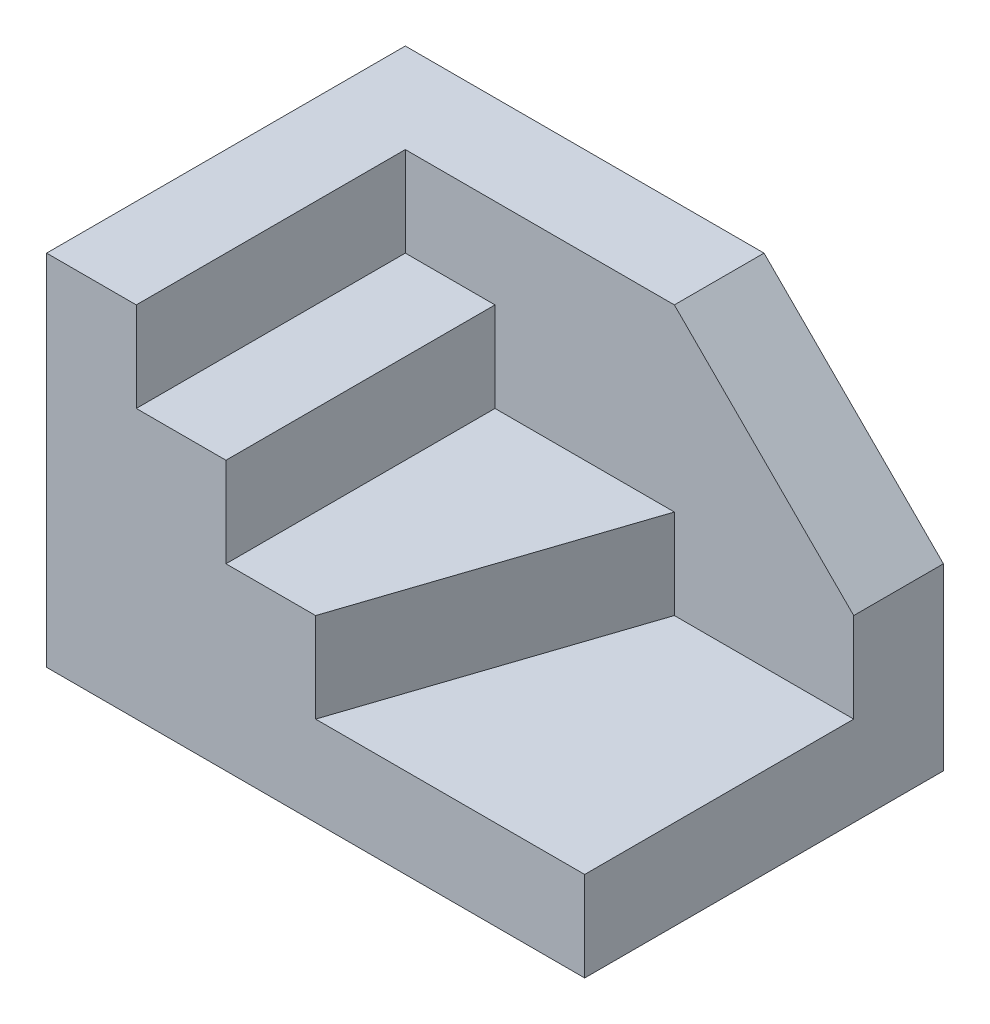
ISO-10303-21;
HEADER;
FILE_DESCRIPTION(('STEP AP214'),'2;1');
FILE_NAME('part.step','',(''),(''),'','','');
FILE_SCHEMA(('AUTOMOTIVE_DESIGN { 1 0 10303 214 1 1 1 1 }'));
ENDSEC;
DATA;
#1=APPLICATION_CONTEXT('core data for automotive mechanical design processes');
#2=APPLICATION_PROTOCOL_DEFINITION('international standard','automotive_design',2000,#1);
#3=PRODUCT_CONTEXT('',#1,'mechanical');
#4=PRODUCT('Part','Part','',(#3));
#5=PRODUCT_RELATED_PRODUCT_CATEGORY('part','',(#4));
#6=PRODUCT_DEFINITION_FORMATION('','',#4);
#7=PRODUCT_DEFINITION_CONTEXT('part definition',#1,'design');
#8=PRODUCT_DEFINITION('design','',#6,#7);
#9=PRODUCT_DEFINITION_SHAPE('','',#8);
#10=(LENGTH_UNIT() NAMED_UNIT(*) SI_UNIT(.MILLI.,.METRE.));
#11=(NAMED_UNIT(*) PLANE_ANGLE_UNIT() SI_UNIT($,.RADIAN.));
#12=(NAMED_UNIT(*) SI_UNIT($,.STERADIAN.) SOLID_ANGLE_UNIT());
#13=UNCERTAINTY_MEASURE_WITH_UNIT(LENGTH_MEASURE(1.E-05),#10,'distance_accuracy_value','');
#14=(GEOMETRIC_REPRESENTATION_CONTEXT(3) GLOBAL_UNCERTAINTY_ASSIGNED_CONTEXT((#13)) GLOBAL_UNIT_ASSIGNED_CONTEXT((#10,
#11,#12)) REPRESENTATION_CONTEXT('',''));
#15=CARTESIAN_POINT('',(0.,0.,0.));
#16=DIRECTION('',(0.,0.,1.));
#17=DIRECTION('',(1.,0.,0.));
#18=AXIS2_PLACEMENT_3D('',#15,#16,#17);
#19=CARTESIAN_POINT('',(-30.,10.,-20.));
#20=DIRECTION('',(1.,0.,0.));
#21=DIRECTION('',(0.,0.,-1.));
#22=AXIS2_PLACEMENT_3D('',#19,#20,#21);
#23=PLANE('',#22);
#24=DIRECTION('',(0.,-1.,0.));
#25=VECTOR('',#24,1.);
#26=CARTESIAN_POINT('',(-30.,10.,20.));
#27=LINE('',#26,#25);
#28=CARTESIAN_POINT('',(-30.,40.,20.));
#29=VERTEX_POINT('',#28);
#30=CARTESIAN_POINT('',(-30.,0.,20.));
#31=VERTEX_POINT('',#30);
#32=EDGE_CURVE('E213',#29,#31,#27,.T.);
#33=ORIENTED_EDGE('',*,*,#32,.F.);
#34=DIRECTION('',(0.,0.,1.));
#35=VECTOR('',#34,1.);
#36=CARTESIAN_POINT('',(-30.,40.,-62.4264068711929));
#37=LINE('',#36,#35);
#38=CARTESIAN_POINT('',(-30.,40.,-20.));
#39=VERTEX_POINT('',#38);
#40=EDGE_CURVE('E169',#39,#29,#37,.T.);
#41=ORIENTED_EDGE('',*,*,#40,.F.);
#42=DIRECTION('',(0.,-1.,0.));
#43=VECTOR('',#42,1.);
#44=CARTESIAN_POINT('',(-30.,10.,-20.));
#45=LINE('',#44,#43);
#46=CARTESIAN_POINT('',(-30.,0.,-20.));
#47=VERTEX_POINT('',#46);
#48=EDGE_CURVE('E196',#39,#47,#45,.T.);
#49=ORIENTED_EDGE('',*,*,#48,.T.);
#50=DIRECTION('',(0.,0.,1.));
#51=VECTOR('',#50,1.);
#52=CARTESIAN_POINT('',(-30.,0.,-20.));
#53=LINE('',#52,#51);
#54=EDGE_CURVE('E170',#47,#31,#53,.T.);
#55=ORIENTED_EDGE('',*,*,#54,.T.);
#56=EDGE_LOOP('',(#33,#41,#49,#55));
#57=FACE_BOUND('',#56,.T.);
#58=ADVANCED_FACE('F41',(#57),#23,.F.);
#59=CARTESIAN_POINT('',(30.,10.,20.));
#60=DIRECTION('',(0.,0.,-1.));
#61=DIRECTION('',(-1.,0.,0.));
#62=AXIS2_PLACEMENT_3D('',#59,#60,#61);
#63=PLANE('',#62);
#64=DIRECTION('',(1.,0.,0.));
#65=VECTOR('',#64,1.);
#66=CARTESIAN_POINT('',(30.,10.,20.));
#67=LINE('',#66,#65);
#68=CARTESIAN_POINT('',(0.,10.,20.));
#69=VERTEX_POINT('',#68);
#70=CARTESIAN_POINT('',(30.,10.,20.));
#71=VERTEX_POINT('',#70);
#72=EDGE_CURVE('E191',#69,#71,#67,.T.);
#73=ORIENTED_EDGE('',*,*,#72,.F.);
#74=DIRECTION('',(0.,-1.,0.));
#75=VECTOR('',#74,1.);
#76=CARTESIAN_POINT('',(0.,20.,20.));
#77=LINE('',#76,#75);
#78=CARTESIAN_POINT('',(0.,20.,20.));
#79=VERTEX_POINT('',#78);
#80=EDGE_CURVE('E163',#79,#69,#77,.T.);
#81=ORIENTED_EDGE('',*,*,#80,.F.);
#82=DIRECTION('',(1.,0.,0.));
#83=VECTOR('',#82,1.);
#84=CARTESIAN_POINT('',(-9.99999999999999,20.,20.));
#85=LINE('',#84,#83);
#86=CARTESIAN_POINT('',(-9.99999999999999,20.,20.));
#87=VERTEX_POINT('',#86);
#88=EDGE_CURVE('E149',#87,#79,#85,.T.);
#89=ORIENTED_EDGE('',*,*,#88,.F.);
#90=DIRECTION('',(0.,-1.,0.));
#91=VECTOR('',#90,1.);
#92=CARTESIAN_POINT('',(-9.99999999999999,30.,20.));
#93=LINE('',#92,#91);
#94=CARTESIAN_POINT('',(-9.99999999999999,30.,20.));
#95=VERTEX_POINT('',#94);
#96=EDGE_CURVE('E173',#95,#87,#93,.T.);
#97=ORIENTED_EDGE('',*,*,#96,.F.);
#98=DIRECTION('',(1.,0.,0.));
#99=VECTOR('',#98,1.);
#100=CARTESIAN_POINT('',(-20.,30.,20.));
#101=LINE('',#100,#99);
#102=CARTESIAN_POINT('',(-20.,30.,20.));
#103=VERTEX_POINT('',#102);
#104=EDGE_CURVE('E175',#103,#95,#101,.T.);
#105=ORIENTED_EDGE('',*,*,#104,.F.);
#106=DIRECTION('',(0.,-1.,0.));
#107=VECTOR('',#106,1.);
#108=CARTESIAN_POINT('',(-20.,40.,20.));
#109=LINE('',#108,#107);
#110=CARTESIAN_POINT('',(-20.,40.,20.));
#111=VERTEX_POINT('',#110);
#112=EDGE_CURVE('E176',#111,#103,#109,.T.);
#113=ORIENTED_EDGE('',*,*,#112,.F.);
#114=DIRECTION('',(1.,0.,0.));
#115=VECTOR('',#114,1.);
#116=CARTESIAN_POINT('',(-30.,40.,20.));
#117=LINE('',#116,#115);
#118=EDGE_CURVE('E177',#29,#111,#117,.T.);
#119=ORIENTED_EDGE('',*,*,#118,.F.);
#120=ORIENTED_EDGE('',*,*,#32,.T.);
#121=DIRECTION('',(1.,0.,0.));
#122=VECTOR('',#121,1.);
#123=CARTESIAN_POINT('',(30.,0.,20.));
#124=LINE('',#123,#122);
#125=CARTESIAN_POINT('',(30.,0.,20.));
#126=VERTEX_POINT('',#125);
#127=EDGE_CURVE('E199',#31,#126,#124,.T.);
#128=ORIENTED_EDGE('',*,*,#127,.T.);
#129=DIRECTION('',(0.,-1.,0.));
#130=VECTOR('',#129,1.);
#131=CARTESIAN_POINT('',(30.,10.,20.));
#132=LINE('',#131,#130);
#133=EDGE_CURVE('E209',#71,#126,#132,.T.);
#134=ORIENTED_EDGE('',*,*,#133,.F.);
#135=EDGE_LOOP('',(#73,#81,#89,#97,#105,#113,#119,#120,#128,#134));
#136=FACE_BOUND('',#135,.T.);
#137=ADVANCED_FACE('F248',(#136),#63,.F.);
#138=CARTESIAN_POINT('',(30.,10.,-20.));
#139=DIRECTION('',(-1.,0.,0.));
#140=DIRECTION('',(0.,0.,1.));
#141=AXIS2_PLACEMENT_3D('',#138,#139,#140);
#142=PLANE('',#141);
#143=DIRECTION('',(0.,-1.,0.));
#144=VECTOR('',#143,1.);
#145=CARTESIAN_POINT('',(30.,10.,-20.));
#146=LINE('',#145,#144);
#147=CARTESIAN_POINT('',(30.,19.9999999999999,-20.));
#148=VERTEX_POINT('',#147);
#149=CARTESIAN_POINT('',(30.,0.,-20.));
#150=VERTEX_POINT('',#149);
#151=EDGE_CURVE('E208',#148,#150,#146,.T.);
#152=ORIENTED_EDGE('',*,*,#151,.F.);
#153=DIRECTION('',(0.,0.,1.));
#154=VECTOR('',#153,1.);
#155=CARTESIAN_POINT('',(30.,19.9999999999999,-20.));
#156=LINE('',#155,#154);
#157=CARTESIAN_POINT('',(30.,19.9999999999999,-10.));
#158=VERTEX_POINT('',#157);
#159=EDGE_CURVE('E49',#148,#158,#156,.T.);
#160=ORIENTED_EDGE('',*,*,#159,.T.);
#161=DIRECTION('',(0.,-1.,0.));
#162=VECTOR('',#161,1.);
#163=CARTESIAN_POINT('',(30.,0.,-10.));
#164=LINE('',#163,#162);
#165=CARTESIAN_POINT('',(30.,10.,-10.));
#166=VERTEX_POINT('',#165);
#167=EDGE_CURVE('E144',#158,#166,#164,.T.);
#168=ORIENTED_EDGE('',*,*,#167,.T.);
#169=DIRECTION('',(0.,0.,-1.));
#170=VECTOR('',#169,1.);
#171=CARTESIAN_POINT('',(30.,10.,-20.));
#172=LINE('',#171,#170);
#173=EDGE_CURVE('E193',#71,#166,#172,.T.);
#174=ORIENTED_EDGE('',*,*,#173,.F.);
#175=ORIENTED_EDGE('',*,*,#133,.T.);
#176=DIRECTION('',(0.,0.,-1.));
#177=VECTOR('',#176,1.);
#178=CARTESIAN_POINT('',(30.,0.,-20.));
#179=LINE('',#178,#177);
#180=EDGE_CURVE('E205',#126,#150,#179,.T.);
#181=ORIENTED_EDGE('',*,*,#180,.T.);
#182=EDGE_LOOP('',(#152,#160,#168,#174,#175,#181));
#183=FACE_BOUND('',#182,.T.);
#184=ADVANCED_FACE('F228',(#183),#142,.F.);
#185=CARTESIAN_POINT('',(30.,10.,-20.));
#186=DIRECTION('',(0.,0.,1.));
#187=DIRECTION('',(1.,0.,0.));
#188=AXIS2_PLACEMENT_3D('',#185,#186,#187);
#189=PLANE('',#188);
#190=DIRECTION('',(-1.,0.,0.));
#191=VECTOR('',#190,1.);
#192=CARTESIAN_POINT('',(-30.,40.,-20.));
#193=LINE('',#192,#191);
#194=CARTESIAN_POINT('',(9.99999999999999,40.,-20.));
#195=VERTEX_POINT('',#194);
#196=EDGE_CURVE('E164',#195,#39,#193,.T.);
#197=ORIENTED_EDGE('',*,*,#196,.F.);
#198=DIRECTION('',(-0.707106781186547,0.707106781186549,0.));
#199=VECTOR('',#198,1.);
#200=CARTESIAN_POINT('',(9.99999999999999,40.,-20.));
#201=LINE('',#200,#199);
#202=EDGE_CURVE('E218',#195,#148,#201,.F.);
#203=ORIENTED_EDGE('',*,*,#202,.T.);
#204=ORIENTED_EDGE('',*,*,#151,.T.);
#205=DIRECTION('',(-1.,0.,0.));
#206=VECTOR('',#205,1.);
#207=CARTESIAN_POINT('',(30.,0.,-20.));
#208=LINE('',#207,#206);
#209=EDGE_CURVE('E192',#150,#47,#208,.T.);
#210=ORIENTED_EDGE('',*,*,#209,.T.);
#211=ORIENTED_EDGE('',*,*,#48,.F.);
#212=EDGE_LOOP('',(#197,#203,#204,#210,#211));
#213=FACE_BOUND('',#212,.T.);
#214=ADVANCED_FACE('F225',(#213),#189,.F.);
#215=CARTESIAN_POINT('',(0.,10.,0.));
#216=DIRECTION('',(0.,-1.,0.));
#217=DIRECTION('',(0.,0.,-1.));
#218=AXIS2_PLACEMENT_3D('',#215,#216,#217);
#219=PLANE('',#218);
#220=DIRECTION('',(-1.,0.,0.));
#221=VECTOR('',#220,1.);
#222=CARTESIAN_POINT('',(0.,10.,-10.));
#223=LINE('',#222,#221);
#224=CARTESIAN_POINT('',(10.,10.,-10.));
#225=VERTEX_POINT('',#224);
#226=EDGE_CURVE('E139',#166,#225,#223,.T.);
#227=ORIENTED_EDGE('',*,*,#226,.T.);
#228=DIRECTION('',(0.316227766016838,0.,-0.948683298050514));
#229=VECTOR('',#228,1.);
#230=CARTESIAN_POINT('',(10.,10.,-9.99999999999999));
#231=LINE('',#230,#229);
#232=EDGE_CURVE('E145',#69,#225,#231,.T.);
#233=ORIENTED_EDGE('',*,*,#232,.F.);
#234=ORIENTED_EDGE('',*,*,#72,.T.);
#235=ORIENTED_EDGE('',*,*,#173,.T.);
#236=EDGE_LOOP('',(#227,#233,#234,#235));
#237=FACE_BOUND('',#236,.T.);
#238=ADVANCED_FACE('F251',(#237),#219,.F.);
#239=CARTESIAN_POINT('',(0.,0.,0.));
#240=DIRECTION('',(0.,-1.,0.));
#241=DIRECTION('',(0.,0.,-1.));
#242=AXIS2_PLACEMENT_3D('',#239,#240,#241);
#243=PLANE('',#242);
#244=ORIENTED_EDGE('',*,*,#127,.F.);
#245=ORIENTED_EDGE('',*,*,#54,.F.);
#246=ORIENTED_EDGE('',*,*,#209,.F.);
#247=ORIENTED_EDGE('',*,*,#180,.F.);
#248=EDGE_LOOP('',(#244,#245,#246,#247));
#249=FACE_BOUND('',#248,.T.);
#250=ADVANCED_FACE('F258',(#249),#243,.T.);
#251=CARTESIAN_POINT('',(-9.99999999999999,20.,-62.4264068711929));
#252=DIRECTION('',(0.,-1.,0.));
#253=DIRECTION('',(0.,0.,-1.));
#254=AXIS2_PLACEMENT_3D('',#251,#252,#253);
#255=PLANE('',#254);
#256=ORIENTED_EDGE('',*,*,#88,.T.);
#257=DIRECTION('',(0.316227766016838,0.,-0.948683298050514));
#258=VECTOR('',#257,1.);
#259=CARTESIAN_POINT('',(10.,20.,-9.99999999999999));
#260=LINE('',#259,#258);
#261=CARTESIAN_POINT('',(10.,20.,-9.99999999999999));
#262=VERTEX_POINT('',#261);
#263=EDGE_CURVE('E141',#79,#262,#260,.T.);
#264=ORIENTED_EDGE('',*,*,#263,.T.);
#265=DIRECTION('',(-1.,0.,0.));
#266=VECTOR('',#265,1.);
#267=CARTESIAN_POINT('',(-9.99999999999998,20.,-10.));
#268=LINE('',#267,#266);
#269=CARTESIAN_POINT('',(-9.99999999999999,20.,-10.));
#270=VERTEX_POINT('',#269);
#271=EDGE_CURVE('E129',#262,#270,#268,.T.);
#272=ORIENTED_EDGE('',*,*,#271,.T.);
#273=DIRECTION('',(0.,0.,1.));
#274=VECTOR('',#273,1.);
#275=CARTESIAN_POINT('',(-9.99999999999999,20.,-62.4264068711929));
#276=LINE('',#275,#274);
#277=EDGE_CURVE('E181',#270,#87,#276,.T.);
#278=ORIENTED_EDGE('',*,*,#277,.T.);
#279=EDGE_LOOP('',(#256,#264,#272,#278));
#280=FACE_BOUND('',#279,.T.);
#281=ADVANCED_FACE('F150',(#280),#255,.F.);
#282=CARTESIAN_POINT('',(-9.99999999999999,30.,-62.4264068711929));
#283=DIRECTION('',(-1.,0.,0.));
#284=DIRECTION('',(0.,0.,1.));
#285=AXIS2_PLACEMENT_3D('',#282,#283,#284);
#286=PLANE('',#285);
#287=ORIENTED_EDGE('',*,*,#277,.F.);
#288=DIRECTION('',(0.,1.,0.));
#289=VECTOR('',#288,1.);
#290=CARTESIAN_POINT('',(-9.99999999999999,30.,-10.));
#291=LINE('',#290,#289);
#292=CARTESIAN_POINT('',(-9.99999999999999,30.,-10.));
#293=VERTEX_POINT('',#292);
#294=EDGE_CURVE('E134',#270,#293,#291,.T.);
#295=ORIENTED_EDGE('',*,*,#294,.T.);
#296=DIRECTION('',(0.,0.,1.));
#297=VECTOR('',#296,1.);
#298=CARTESIAN_POINT('',(-9.99999999999999,30.,-62.4264068711929));
#299=LINE('',#298,#297);
#300=EDGE_CURVE('E190',#293,#95,#299,.T.);
#301=ORIENTED_EDGE('',*,*,#300,.T.);
#302=ORIENTED_EDGE('',*,*,#96,.T.);
#303=EDGE_LOOP('',(#287,#295,#301,#302));
#304=FACE_BOUND('',#303,.T.);
#305=ADVANCED_FACE('F249',(#304),#286,.F.);
#306=CARTESIAN_POINT('',(-20.,30.,-62.4264068711929));
#307=DIRECTION('',(0.,-1.,0.));
#308=DIRECTION('',(0.,0.,-1.));
#309=AXIS2_PLACEMENT_3D('',#306,#307,#308);
#310=PLANE('',#309);
#311=ORIENTED_EDGE('',*,*,#300,.F.);
#312=DIRECTION('',(-1.,0.,0.));
#313=VECTOR('',#312,1.);
#314=CARTESIAN_POINT('',(-20.,30.,-10.));
#315=LINE('',#314,#313);
#316=CARTESIAN_POINT('',(-20.,30.,-10.));
#317=VERTEX_POINT('',#316);
#318=EDGE_CURVE('E159',#293,#317,#315,.T.);
#319=ORIENTED_EDGE('',*,*,#318,.T.);
#320=DIRECTION('',(0.,0.,1.));
#321=VECTOR('',#320,1.);
#322=CARTESIAN_POINT('',(-20.,30.,-62.4264068711929));
#323=LINE('',#322,#321);
#324=EDGE_CURVE('E189',#317,#103,#323,.T.);
#325=ORIENTED_EDGE('',*,*,#324,.T.);
#326=ORIENTED_EDGE('',*,*,#104,.T.);
#327=EDGE_LOOP('',(#311,#319,#325,#326));
#328=FACE_BOUND('',#327,.T.);
#329=ADVANCED_FACE('F242',(#328),#310,.F.);
#330=CARTESIAN_POINT('',(-20.,40.,-62.4264068711929));
#331=DIRECTION('',(-1.,0.,0.));
#332=DIRECTION('',(0.,0.,1.));
#333=AXIS2_PLACEMENT_3D('',#330,#331,#332);
#334=PLANE('',#333);
#335=ORIENTED_EDGE('',*,*,#324,.F.);
#336=DIRECTION('',(0.,1.,0.));
#337=VECTOR('',#336,1.);
#338=CARTESIAN_POINT('',(-20.,40.,-10.));
#339=LINE('',#338,#337);
#340=CARTESIAN_POINT('',(-20.,40.,-9.99999999999999));
#341=VERTEX_POINT('',#340);
#342=EDGE_CURVE('E158',#317,#341,#339,.T.);
#343=ORIENTED_EDGE('',*,*,#342,.T.);
#344=DIRECTION('',(0.,0.,1.));
#345=VECTOR('',#344,1.);
#346=CARTESIAN_POINT('',(-20.,40.,-62.4264068711929));
#347=LINE('',#346,#345);
#348=EDGE_CURVE('E183',#341,#111,#347,.T.);
#349=ORIENTED_EDGE('',*,*,#348,.T.);
#350=ORIENTED_EDGE('',*,*,#112,.T.);
#351=EDGE_LOOP('',(#335,#343,#349,#350));
#352=FACE_BOUND('',#351,.T.);
#353=ADVANCED_FACE('F239',(#352),#334,.F.);
#354=CARTESIAN_POINT('',(-30.,40.,-62.4264068711929));
#355=DIRECTION('',(0.,-1.,0.));
#356=DIRECTION('',(0.,0.,-1.));
#357=AXIS2_PLACEMENT_3D('',#354,#355,#356);
#358=PLANE('',#357);
#359=DIRECTION('',(1.,0.,0.));
#360=VECTOR('',#359,1.);
#361=CARTESIAN_POINT('',(30.,40.,-10.));
#362=LINE('',#361,#360);
#363=CARTESIAN_POINT('',(9.99999999999999,40.,-10.));
#364=VERTEX_POINT('',#363);
#365=EDGE_CURVE('E154',#341,#364,#362,.T.);
#366=ORIENTED_EDGE('',*,*,#365,.T.);
#367=DIRECTION('',(0.,0.,-1.));
#368=VECTOR('',#367,1.);
#369=CARTESIAN_POINT('',(9.99999999999998,40.,-62.4264068711929));
#370=LINE('',#369,#368);
#371=EDGE_CURVE('E216',#364,#195,#370,.T.);
#372=ORIENTED_EDGE('',*,*,#371,.T.);
#373=ORIENTED_EDGE('',*,*,#196,.T.);
#374=ORIENTED_EDGE('',*,*,#40,.T.);
#375=ORIENTED_EDGE('',*,*,#118,.T.);
#376=ORIENTED_EDGE('',*,*,#348,.F.);
#377=EDGE_LOOP('',(#366,#372,#373,#374,#375,#376));
#378=FACE_BOUND('',#377,.T.);
#379=ADVANCED_FACE('F233',(#378),#358,.F.);
#380=CARTESIAN_POINT('',(0.,0.,-10.));
#381=DIRECTION('',(0.,0.,1.));
#382=DIRECTION('',(1.,0.,0.));
#383=AXIS2_PLACEMENT_3D('',#380,#381,#382);
#384=PLANE('',#383);
#385=ORIENTED_EDGE('',*,*,#271,.F.);
#386=DIRECTION('',(0.,1.,0.));
#387=VECTOR('',#386,1.);
#388=CARTESIAN_POINT('',(10.,-26.0555127546399,-9.99999999999999));
#389=LINE('',#388,#387);
#390=EDGE_CURVE('E60',#225,#262,#389,.T.);
#391=ORIENTED_EDGE('',*,*,#390,.F.);
#392=ORIENTED_EDGE('',*,*,#226,.F.);
#393=ORIENTED_EDGE('',*,*,#167,.F.);
#394=DIRECTION('',(0.707106781186547,-0.707106781186549,0.));
#395=VECTOR('',#394,1.);
#396=CARTESIAN_POINT('',(25.,24.9999999999999,-10.));
#397=LINE('',#396,#395);
#398=EDGE_CURVE('E11',#158,#364,#397,.F.);
#399=ORIENTED_EDGE('',*,*,#398,.T.);
#400=ORIENTED_EDGE('',*,*,#365,.F.);
#401=ORIENTED_EDGE('',*,*,#342,.F.);
#402=ORIENTED_EDGE('',*,*,#318,.F.);
#403=ORIENTED_EDGE('',*,*,#294,.F.);
#404=EDGE_LOOP('',(#385,#391,#392,#393,#399,#400,#401,#402,#403));
#405=FACE_BOUND('',#404,.T.);
#406=ADVANCED_FACE('F128',(#405),#384,.T.);
#407=CARTESIAN_POINT('',(9.99999999999998,40.,-62.4264068711929));
#408=DIRECTION('',(-0.707106781186549,-0.707106781186547,0.));
#409=DIRECTION('',(0.,0.,-1.));
#410=AXIS2_PLACEMENT_3D('',#407,#408,#409);
#411=PLANE('',#410);
#412=ORIENTED_EDGE('',*,*,#398,.F.);
#413=ORIENTED_EDGE('',*,*,#159,.F.);
#414=ORIENTED_EDGE('',*,*,#202,.F.);
#415=ORIENTED_EDGE('',*,*,#371,.F.);
#416=EDGE_LOOP('',(#412,#413,#414,#415));
#417=FACE_BOUND('',#416,.T.);
#418=ADVANCED_FACE('F42',(#417),#411,.F.);
#419=CARTESIAN_POINT('',(10.,-26.0555127546399,-9.99999999999999));
#420=DIRECTION('',(0.948683298050514,0.,0.316227766016838));
#421=DIRECTION('',(0.316227766016838,0.,-0.948683298050514));
#422=AXIS2_PLACEMENT_3D('',#419,#420,#421);
#423=PLANE('',#422);
#424=ORIENTED_EDGE('',*,*,#80,.T.);
#425=ORIENTED_EDGE('',*,*,#232,.T.);
#426=ORIENTED_EDGE('',*,*,#390,.T.);
#427=ORIENTED_EDGE('',*,*,#263,.F.);
#428=EDGE_LOOP('',(#424,#425,#426,#427));
#429=FACE_BOUND('',#428,.T.);
#430=ADVANCED_FACE('F142',(#429),#423,.T.);
#431=CLOSED_SHELL('',(#58,#137,#184,#214,#238,#250,#281,#305,#329,#353,#379,#406,#418,#430));
#432=MANIFOLD_SOLID_BREP('B2',#431);
#433=ADVANCED_BREP_SHAPE_REPRESENTATION('',(#18,#432),#14);
#434=SHAPE_DEFINITION_REPRESENTATION(#9,#433);
ENDSEC;
END-ISO-10303-21;
